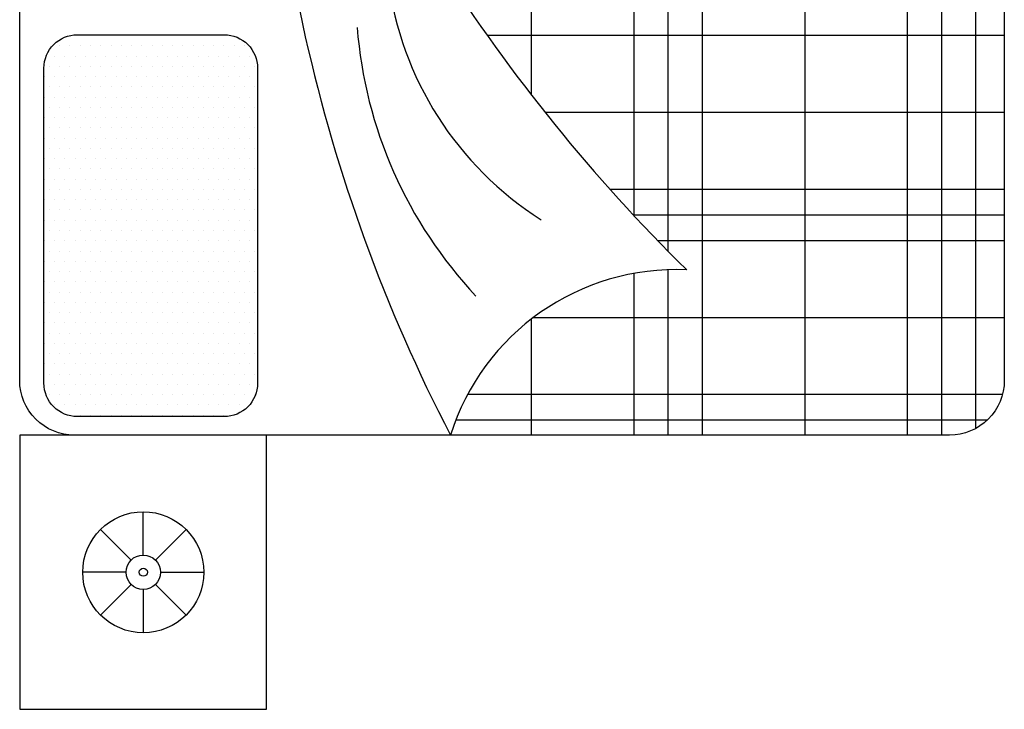
# Model space of a CAD drawing. Units: inches. Extents: x 528 to 2520, y -151 to 1354.
# Tile 18 of 41: x 1137 to 1192, y 1151 to 1189. Entities that reach past the tile are written whole.
import ezdxf

# ---------------------------------------------------------------- set-up
doc = ezdxf.new("R2010")
doc.units = ezdxf.units.IN
doc.header["$MEASUREMENT"] = 0
doc.layers.add('A-FURN', color=8, linetype='Continuous', lineweight=18)
doc.layers.add('BLOCK', color=6, linetype='Continuous')

# ---------------------------------------------------------------- blocks, each defined once
blk = doc.blocks.new('*X15')
at = {"color": 0}
for p, q in [((276.598, 451.25), (280.51, 451.25)), ((275.455, 450.625), (280.51, 450.625)), ((274.411, 450), (280.51, 450)), ((265.51, 448.125), (267.634, 448.125)), ((271.723, 448.125), (280.51, 448.125)), ((265.51, 446.25), (268.465, 446.25)), ((269.519, 446.25), (280.51, 446.25)), ((265.51, 445.625), (268.531, 445.625)), ((268.866, 445.625), (280.51, 445.625)), ((265.51, 445), (280.51, 445)), ((265.51, 443.125), (280.51, 443.125)), ((265.51, 441.25), (280.51, 441.25)), ((265.51, 440.625), (280.51, 440.625)), ((265.634, 440), (280.386, 440))]:
    blk.add_line(p, q, dxfattribs=at)
blk = doc.blocks.new('*X16')
at = {"color": 0}
for p, q in [((280.312, 439.886), (280.312, 452.896)), ((278.906, 439.482), (278.906, 452.338)), ((277.5, 439.482), (277.5, 451.702)), ((277.031, 439.482), (277.031, 451.471)), ((276.562, 439.482), (276.562, 451.231)), ((275.156, 439.482), (275.156, 450.451)), ((265.781, 439.797), (265.781, 449.511)), ((273.75, 439.482), (273.75, 449.576)), ((266.25, 439.517), (266.25, 449.296)), ((273.281, 439.482), (273.281, 449.261)), ((272.812, 439.482), (272.812, 448.934)), ((267.656, 439.482), (267.656, 448.095)), ((271.406, 439.482), (271.406, 447.876)), ((270, 439.482), (270, 446.689)), ((269.531, 439.482), (269.531, 446.262)), ((269.062, 439.482), (269.062, 445.817))]:
    blk.add_line(p, q, dxfattribs=at)
blk = doc.blocks.new('*X17')
at = {"color": 0}
for p, q in [((266.4375, 457.03125), (266.4375, 457.03125)), ((266.8125, 457.03125), (266.8125, 457.03125)), ((267.1875, 457.03125), (267.1875, 457.03125)), ((267.5625, 457.03125), (267.5625, 457.03125)), ((267.9375, 457.03125), (267.9375, 457.03125)), ((268.3125, 457.03125), (268.3125, 457.03125)), ((268.6875, 457.03125), (268.6875, 457.03125)), ((269.0625, 457.03125), (269.0625, 457.03125)), ((269.4375, 457.03125), (269.4375, 457.03125)), ((269.8125, 457.03125), (269.8125, 457.03125)), ((270.1875, 457.03125), (270.1875, 457.03125)), ((270.5625, 457.03125), (270.5625, 457.03125)), ((270.9375, 457.03125), (270.9375, 457.03125)), ((271.3125, 457.03125), (271.3125, 457.03125)), ((271.6875, 457.03125), (271.6875, 457.03125)), ((272.0625, 457.03125), (272.0625, 457.03125)), ((266.0625, 456.84375), (266.0625, 456.84375)), ((266.25, 456.9375), (266.25, 456.9375)), ((266.4375, 456.84375), (266.4375, 456.84375)), ((266.625, 456.9375), (266.625, 456.9375)), ((266.8125, 456.84375), (266.8125, 456.84375)), ((267, 456.9375), (267, 456.9375)), ((267.1875, 456.84375), (267.1875, 456.84375)), ((267.375, 456.9375), (267.375, 456.9375)), ((267.5625, 456.84375), (267.5625, 456.84375)), ((267.75, 456.9375), (267.75, 456.9375)), ((267.9375, 456.84375), (267.9375, 456.84375)), ((268.125, 456.9375), (268.125, 456.9375)), ((268.3125, 456.84375), (268.3125, 456.84375)), ((268.5, 456.9375), (268.5, 456.9375)), ((268.6875, 456.84375), (268.6875, 456.84375)), ((268.875, 456.9375), (268.875, 456.9375)), ((269.0625, 456.84375), (269.0625, 456.84375)), ((269.25, 456.9375), (269.25, 456.9375)), ((269.4375, 456.84375), (269.4375, 456.84375)), ((269.625, 456.9375), (269.625, 456.9375)), ((269.8125, 456.84375), (269.8125, 456.84375)), ((270, 456.9375), (270, 456.9375)), ((270.1875, 456.84375), (270.1875, 456.84375)), ((270.375, 456.9375), (270.375, 456.9375)), ((270.5625, 456.84375), (270.5625, 456.84375)), ((270.75, 456.9375), (270.75, 456.9375)), ((270.9375, 456.84375), (270.9375, 456.84375)), ((271.125, 456.9375), (271.125, 456.9375)), ((271.3125, 456.84375), (271.3125, 456.84375)), ((271.5, 456.9375), (271.5, 456.9375)), ((271.6875, 456.84375), (271.6875, 456.84375)), ((271.875, 456.9375), (271.875, 456.9375)), ((272.0625, 456.84375), (272.0625, 456.84375)), ((272.25, 456.9375), (272.25, 456.9375)), ((272.4375, 456.84375), (272.4375, 456.84375)), ((266.25, 456.75), (266.25, 456.75)), ((266.625, 456.75), (266.625, 456.75)), ((267, 456.75), (267, 456.75)), ((267.375, 456.75), (267.375, 456.75)), ((267.75, 456.75), (267.75, 456.75)), ((268.125, 456.75), (268.125, 456.75)), ((268.5, 456.75), (268.5, 456.75)), ((268.875, 456.75), (268.875, 456.75)), ((269.25, 456.75), (269.25, 456.75)), ((269.625, 456.75), (269.625, 456.75)), ((270, 456.75), (270, 456.75)), ((270.375, 456.75), (270.375, 456.75)), ((270.75, 456.75), (270.75, 456.75)), ((271.125, 456.75), (271.125, 456.75)), ((271.5, 456.75), (271.5, 456.75)), ((271.875, 456.75), (271.875, 456.75)), ((272.25, 456.75), (272.25, 456.75)), ((272.625, 456.75), (272.625, 456.75)), ((265.875, 456.5625), (265.875, 456.5625)), ((266.0625, 456.65625), (266.0625, 456.65625)), ((266.25, 456.5625), (266.25, 456.5625)), ((266.4375, 456.65625), (266.4375, 456.65625)), ((266.625, 456.5625), (266.625, 456.5625)), ((266.8125, 456.65625), (266.8125, 456.65625)), ((267, 456.5625), (267, 456.5625)), ((267.1875, 456.65625), (267.1875, 456.65625)), ((267.375, 456.5625), (267.375, 456.5625)), ((267.5625, 456.65625), (267.5625, 456.65625)), ((267.75, 456.5625), (267.75, 456.5625)), ((267.9375, 456.65625), (267.9375, 456.65625)), ((268.125, 456.5625), (268.125, 456.5625)), ((268.3125, 456.65625), (268.3125, 456.65625)), ((268.5, 456.5625), (268.5, 456.5625)), ((268.6875, 456.65625), (268.6875, 456.65625)), ((268.875, 456.5625), (268.875, 456.5625)), ((269.0625, 456.65625), (269.0625, 456.65625)), ((269.25, 456.5625), (269.25, 456.5625)), ((269.4375, 456.65625), (269.4375, 456.65625)), ((269.625, 456.5625), (269.625, 456.5625)), ((269.8125, 456.65625), (269.8125, 456.65625)), ((270, 456.5625), (270, 456.5625)), ((270.1875, 456.65625), (270.1875, 456.65625)), ((270.375, 456.5625), (270.375, 456.5625)), ((270.5625, 456.65625), (270.5625, 456.65625)), ((270.75, 456.5625), (270.75, 456.5625)), ((270.9375, 456.65625), (270.9375, 456.65625)), ((271.125, 456.5625), (271.125, 456.5625)), ((271.3125, 456.65625), (271.3125, 456.65625)), ((271.5, 456.5625), (271.5, 456.5625)), ((271.6875, 456.65625), (271.6875, 456.65625)), ((271.875, 456.5625), (271.875, 456.5625)), ((272.0625, 456.65625), (272.0625, 456.65625)), ((272.25, 456.5625), (272.25, 456.5625)), ((272.4375, 456.65625), (272.4375, 456.65625)), ((272.625, 456.5625), (272.625, 456.5625)), ((265.875, 456.375), (265.875, 456.375)), ((266.0625, 456.46875), (266.0625, 456.46875)), ((266.25, 456.375), (266.25, 456.375)), ((266.4375, 456.46875), (266.4375, 456.46875)), ((266.625, 456.375), (266.625, 456.375)), ((266.8125, 456.46875), (266.8125, 456.46875)), ((267, 456.375), (267, 456.375)), ((267.1875, 456.46875), (267.1875, 456.46875)), ((267.375, 456.375), (267.375, 456.375)), ((267.5625, 456.46875), (267.5625, 456.46875)), ((267.75, 456.375), (267.75, 456.375)), ((267.9375, 456.46875), (267.9375, 456.46875)), ((268.125, 456.375), (268.125, 456.375)), ((268.3125, 456.46875), (268.3125, 456.46875)), ((268.5, 456.375), (268.5, 456.375)), ((268.6875, 456.46875), (268.6875, 456.46875)), ((268.875, 456.375), (268.875, 456.375)), ((269.0625, 456.46875), (269.0625, 456.46875)), ((269.25, 456.375), (269.25, 456.375)), ((269.4375, 456.46875), (269.4375, 456.46875)), ((269.625, 456.375), (269.625, 456.375)), ((269.8125, 456.46875), (269.8125, 456.46875)), ((270, 456.375), (270, 456.375)), ((270.1875, 456.46875), (270.1875, 456.46875)), ((270.375, 456.375), (270.375, 456.375)), ((270.5625, 456.46875), (270.5625, 456.46875)), ((270.75, 456.375), (270.75, 456.375)), ((270.9375, 456.46875), (270.9375, 456.46875)), ((271.125, 456.375), (271.125, 456.375)), ((271.3125, 456.46875), (271.3125, 456.46875)), ((271.5, 456.375), (271.5, 456.375)), ((271.6875, 456.46875), (271.6875, 456.46875)), ((271.875, 456.375), (271.875, 456.375)), ((272.0625, 456.46875), (272.0625, 456.46875)), ((272.25, 456.375), (272.25, 456.375)), ((272.4375, 456.46875), (272.4375, 456.46875)), ((272.625, 456.375), (272.625, 456.375)), ((272.8125, 456.46875), (272.8125, 456.46875)), ((265.875, 456.1875), (265.875, 456.1875)), ((266.0625, 456.28125), (266.0625, 456.28125)), ((266.25, 456.1875), (266.25, 456.1875)), ((266.4375, 456.28125), (266.4375, 456.28125)), ((266.625, 456.1875), (266.625, 456.1875)), ((266.8125, 456.28125), (266.8125, 456.28125)), ((267, 456.1875), (267, 456.1875)), ((267.1875, 456.28125), (267.1875, 456.28125)), ((267.375, 456.1875), (267.375, 456.1875)), ((267.5625, 456.28125), (267.5625, 456.28125)), ((267.75, 456.1875), (267.75, 456.1875)), ((267.9375, 456.28125), (267.9375, 456.28125)), ((268.125, 456.1875), (268.125, 456.1875)), ((268.3125, 456.28125), (268.3125, 456.28125)), ((268.5, 456.1875), (268.5, 456.1875)), ((268.6875, 456.28125), (268.6875, 456.28125)), ((268.875, 456.1875), (268.875, 456.1875)), ((269.0625, 456.28125), (269.0625, 456.28125)), ((269.25, 456.1875), (269.25, 456.1875)), ((269.4375, 456.28125), (269.4375, 456.28125)), ((269.625, 456.1875), (269.625, 456.1875)), ((269.8125, 456.28125), (269.8125, 456.28125)), ((270, 456.1875), (270, 456.1875)), ((270.1875, 456.28125), (270.1875, 456.28125)), ((270.375, 456.1875), (270.375, 456.1875)), ((270.5625, 456.28125), (270.5625, 456.28125)), ((270.75, 456.1875), (270.75, 456.1875)), ((270.9375, 456.28125), (270.9375, 456.28125)), ((271.125, 456.1875), (271.125, 456.1875)), ((271.3125, 456.28125), (271.3125, 456.28125)), ((271.5, 456.1875), (271.5, 456.1875)), ((271.6875, 456.28125), (271.6875, 456.28125)), ((271.875, 456.1875), (271.875, 456.1875)), ((272.0625, 456.28125), (272.0625, 456.28125)), ((272.25, 456.1875), (272.25, 456.1875)), ((272.4375, 456.28125), (272.4375, 456.28125)), ((272.625, 456.1875), (272.625, 456.1875)), ((272.8125, 456.28125), (272.8125, 456.28125)), ((265.875, 456), (265.875, 456)), ((266.0625, 456.09375), (266.0625, 456.09375)), ((266.25, 456), (266.25, 456)), ((266.4375, 456.09375), (266.4375, 456.09375)), ((266.625, 456), (266.625, 456)), ((266.8125, 456.09375), (266.8125, 456.09375)), ((267, 456), (267, 456)), ((267.1875, 456.09375), (267.1875, 456.09375)), ((267.375, 456), (267.375, 456)), ((267.5625, 456.09375), (267.5625, 456.09375)), ((267.75, 456), (267.75, 456)), ((267.9375, 456.09375), (267.9375, 456.09375)), ((268.125, 456), (268.125, 456)), ((268.3125, 456.09375), (268.3125, 456.09375)), ((268.5, 456), (268.5, 456)), ((268.6875, 456.09375), (268.6875, 456.09375)), ((268.875, 456), (268.875, 456)), ((269.0625, 456.09375), (269.0625, 456.09375)), ((269.25, 456), (269.25, 456)), ((269.4375, 456.09375), (269.4375, 456.09375)), ((269.625, 456), (269.625, 456)), ((269.8125, 456.09375), (269.8125, 456.09375)), ((270, 456), (270, 456)), ((270.1875, 456.09375), (270.1875, 456.09375)), ((270.375, 456), (270.375, 456)), ((270.5625, 456.09375), (270.5625, 456.09375)), ((270.75, 456), (270.75, 456)), ((270.9375, 456.09375), (270.9375, 456.09375)), ((271.125, 456), (271.125, 456)), ((271.3125, 456.09375), (271.3125, 456.09375)), ((271.5, 456), (271.5, 456)), ((271.6875, 456.09375), (271.6875, 456.09375)), ((271.875, 456), (271.875, 456)), ((272.0625, 456.09375), (272.0625, 456.09375)), ((272.25, 456), (272.25, 456)), ((272.4375, 456.09375), (272.4375, 456.09375)), ((272.625, 456), (272.625, 456)), ((272.8125, 456.09375), (272.8125, 456.09375)), ((265.875, 455.8125), (265.875, 455.8125)), ((266.0625, 455.90625), (266.0625, 455.90625)), ((266.25, 455.8125), (266.25, 455.8125)), ((266.4375, 455.90625), (266.4375, 455.90625)), ((266.625, 455.8125), (266.625, 455.8125)), ((266.8125, 455.90625), (266.8125, 455.90625)), ((267, 455.8125), (267, 455.8125)), ((267.1875, 455.90625), (267.1875, 455.90625)), ((267.375, 455.8125), (267.375, 455.8125)), ((267.5625, 455.90625), (267.5625, 455.90625)), ((267.75, 455.8125), (267.75, 455.8125)), ((267.9375, 455.90625), (267.9375, 455.90625)), ((268.125, 455.8125), (268.125, 455.8125)), ((268.3125, 455.90625), (268.3125, 455.90625)), ((268.5, 455.8125), (268.5, 455.8125)), ((268.6875, 455.90625), (268.6875, 455.90625)), ((268.875, 455.8125), (268.875, 455.8125)), ((269.0625, 455.90625), (269.0625, 455.90625)), ((269.25, 455.8125), (269.25, 455.8125)), ((269.4375, 455.90625), (269.4375, 455.90625)), ((269.625, 455.8125), (269.625, 455.8125)), ((269.8125, 455.90625), (269.8125, 455.90625)), ((270, 455.8125), (270, 455.8125)), ((270.1875, 455.90625), (270.1875, 455.90625)), ((270.375, 455.8125), (270.375, 455.8125)), ((270.5625, 455.90625), (270.5625, 455.90625)), ((270.75, 455.8125), (270.75, 455.8125)), ((270.9375, 455.90625), (270.9375, 455.90625)), ((271.125, 455.8125), (271.125, 455.8125)), ((271.3125, 455.90625), (271.3125, 455.90625)), ((271.5, 455.8125), (271.5, 455.8125)), ((271.6875, 455.90625), (271.6875, 455.90625)), ((271.875, 455.8125), (271.875, 455.8125)), ((272.0625, 455.90625), (272.0625, 455.90625)), ((272.25, 455.8125), (272.25, 455.8125)), ((272.4375, 455.90625), (272.4375, 455.90625)), ((272.625, 455.8125), (272.625, 455.8125)), ((272.8125, 455.90625), (272.8125, 455.90625)), ((265.875, 455.625), (265.875, 455.625)), ((266.0625, 455.71875), (266.0625, 455.71875)), ((266.25, 455.625), (266.25, 455.625)), ((266.4375, 455.71875), (266.4375, 455.71875)), ((266.625, 455.625), (266.625, 455.625)), ((266.8125, 455.71875), (266.8125, 455.71875)), ((267, 455.625), (267, 455.625)), ((267.1875, 455.71875), (267.1875, 455.71875)), ((267.375, 455.625), (267.375, 455.625)), ((267.5625, 455.71875), (267.5625, 455.71875)), ((267.75, 455.625), (267.75, 455.625)), ((267.9375, 455.71875), (267.9375, 455.71875)), ((268.125, 455.625), (268.125, 455.625)), ((268.3125, 455.71875), (268.3125, 455.71875)), ((268.5, 455.625), (268.5, 455.625)), ((268.6875, 455.71875), (268.6875, 455.71875)), ((268.875, 455.625), (268.875, 455.625)), ((269.0625, 455.71875), (269.0625, 455.71875)), ((269.25, 455.625), (269.25, 455.625)), ((269.4375, 455.71875), (269.4375, 455.71875)), ((269.625, 455.625), (269.625, 455.625)), ((269.8125, 455.71875), (269.8125, 455.71875)), ((270, 455.625), (270, 455.625)), ((270.1875, 455.71875), (270.1875, 455.71875)), ((270.375, 455.625), (270.375, 455.625)), ((270.5625, 455.71875), (270.5625, 455.71875)), ((270.75, 455.625), (270.75, 455.625)), ((270.9375, 455.71875), (270.9375, 455.71875)), ((271.125, 455.625), (271.125, 455.625)), ((271.3125, 455.71875), (271.3125, 455.71875)), ((271.5, 455.625), (271.5, 455.625)), ((271.6875, 455.71875), (271.6875, 455.71875)), ((271.875, 455.625), (271.875, 455.625)), ((272.0625, 455.71875), (272.0625, 455.71875)), ((272.25, 455.625), (272.25, 455.625)), ((272.4375, 455.71875), (272.4375, 455.71875)), ((272.625, 455.625), (272.625, 455.625)), ((272.8125, 455.71875), (272.8125, 455.71875)), ((265.875, 455.4375), (265.875, 455.4375)), ((266.0625, 455.53125), (266.0625, 455.53125)), ((266.25, 455.4375), (266.25, 455.4375)), ((266.4375, 455.53125), (266.4375, 455.53125)), ((266.625, 455.4375), (266.625, 455.4375)), ((266.8125, 455.53125), (266.8125, 455.53125)), ((267, 455.4375), (267, 455.4375)), ((267.1875, 455.53125), (267.1875, 455.53125)), ((267.375, 455.4375), (267.375, 455.4375)), ((267.5625, 455.53125), (267.5625, 455.53125)), ((267.75, 455.4375), (267.75, 455.4375)), ((267.9375, 455.53125), (267.9375, 455.53125)), ((268.125, 455.4375), (268.125, 455.4375)), ((268.3125, 455.53125), (268.3125, 455.53125)), ((268.5, 455.4375), (268.5, 455.4375)), ((268.6875, 455.53125), (268.6875, 455.53125)), ((268.875, 455.4375), (268.875, 455.4375)), ((269.0625, 455.53125), (269.0625, 455.53125)), ((269.25, 455.4375), (269.25, 455.4375)), ((269.4375, 455.53125), (269.4375, 455.53125)), ((269.625, 455.4375), (269.625, 455.4375)), ((269.8125, 455.53125), (269.8125, 455.53125)), ((270, 455.4375), (270, 455.4375)), ((270.1875, 455.53125), (270.1875, 455.53125)), ((270.375, 455.4375), (270.375, 455.4375)), ((270.5625, 455.53125), (270.5625, 455.53125)), ((270.75, 455.4375), (270.75, 455.4375)), ((270.9375, 455.53125), (270.9375, 455.53125)), ((271.125, 455.4375), (271.125, 455.4375)), ((271.3125, 455.53125), (271.3125, 455.53125)), ((271.5, 455.4375), (271.5, 455.4375)), ((271.6875, 455.53125), (271.6875, 455.53125)), ((271.875, 455.4375), (271.875, 455.4375)), ((272.0625, 455.53125), (272.0625, 455.53125)), ((272.25, 455.4375), (272.25, 455.4375)), ((272.4375, 455.53125), (272.4375, 455.53125)), ((272.625, 455.4375), (272.625, 455.4375)), ((272.8125, 455.53125), (272.8125, 455.53125)), ((265.875, 455.25), (265.875, 455.25)), ((266.0625, 455.34375), (266.0625, 455.34375)), ((266.25, 455.25), (266.25, 455.25)), ((266.4375, 455.34375), (266.4375, 455.34375)), ((266.625, 455.25), (266.625, 455.25)), ((266.8125, 455.34375), (266.8125, 455.34375)), ((267, 455.25), (267, 455.25)), ((267.1875, 455.34375), (267.1875, 455.34375)), ((267.375, 455.25), (267.375, 455.25)), ((267.5625, 455.34375), (267.5625, 455.34375)), ((267.75, 455.25), (267.75, 455.25)), ((267.9375, 455.34375), (267.9375, 455.34375)), ((268.125, 455.25), (268.125, 455.25)), ((268.3125, 455.34375), (268.3125, 455.34375)), ((268.5, 455.25), (268.5, 455.25)), ((268.6875, 455.34375), (268.6875, 455.34375)), ((268.875, 455.25), (268.875, 455.25)), ((269.0625, 455.34375), (269.0625, 455.34375)), ((269.25, 455.25), (269.25, 455.25)), ((269.4375, 455.34375), (269.4375, 455.34375)), ((269.625, 455.25), (269.625, 455.25)), ((269.8125, 455.34375), (269.8125, 455.34375)), ((270, 455.25), (270, 455.25)), ((270.1875, 455.34375), (270.1875, 455.34375)), ((270.375, 455.25), (270.375, 455.25)), ((270.5625, 455.34375), (270.5625, 455.34375)), ((270.75, 455.25), (270.75, 455.25)), ((270.9375, 455.34375), (270.9375, 455.34375)), ((271.125, 455.25), (271.125, 455.25)), ((271.3125, 455.34375), (271.3125, 455.34375)), ((271.5, 455.25), (271.5, 455.25)), ((271.6875, 455.34375), (271.6875, 455.34375)), ((271.875, 455.25), (271.875, 455.25)), ((272.0625, 455.34375), (272.0625, 455.34375)), ((272.25, 455.25), (272.25, 455.25)), ((272.4375, 455.34375), (272.4375, 455.34375)), ((272.625, 455.25), (272.625, 455.25)), ((272.8125, 455.34375), (272.8125, 455.34375)), ((265.875, 455.0625), (265.875, 455.0625)), ((266.0625, 455.15625), (266.0625, 455.15625)), ((266.25, 455.0625), (266.25, 455.0625)), ((266.4375, 455.15625), (266.4375, 455.15625)), ((266.625, 455.0625), (266.625, 455.0625)), ((266.8125, 455.15625), (266.8125, 455.15625)), ((267, 455.0625), (267, 455.0625)), ((267.1875, 455.15625), (267.1875, 455.15625)), ((267.375, 455.0625), (267.375, 455.0625)), ((267.5625, 455.15625), (267.5625, 455.15625)), ((267.75, 455.0625), (267.75, 455.0625)), ((267.9375, 455.15625), (267.9375, 455.15625)), ((268.125, 455.0625), (268.125, 455.0625)), ((268.3125, 455.15625), (268.3125, 455.15625)), ((268.5, 455.0625), (268.5, 455.0625)), ((268.6875, 455.15625), (268.6875, 455.15625)), ((268.875, 455.0625), (268.875, 455.0625)), ((269.0625, 455.15625), (269.0625, 455.15625)), ((269.25, 455.0625), (269.25, 455.0625)), ((269.4375, 455.15625), (269.4375, 455.15625)), ((269.625, 455.0625), (269.625, 455.0625)), ((269.8125, 455.15625), (269.8125, 455.15625)), ((270, 455.0625), (270, 455.0625)), ((270.1875, 455.15625), (270.1875, 455.15625)), ((270.375, 455.0625), (270.375, 455.0625)), ((270.5625, 455.15625), (270.5625, 455.15625)), ((270.75, 455.0625), (270.75, 455.0625)), ((270.9375, 455.15625), (270.9375, 455.15625)), ((271.125, 455.0625), (271.125, 455.0625)), ((271.3125, 455.15625), (271.3125, 455.15625)), ((271.5, 455.0625), (271.5, 455.0625)), ((271.6875, 455.15625), (271.6875, 455.15625)), ((271.875, 455.0625), (271.875, 455.0625)), ((272.0625, 455.15625), (272.0625, 455.15625)), ((272.25, 455.0625), (272.25, 455.0625)), ((272.4375, 455.15625), (272.4375, 455.15625)), ((272.625, 455.0625), (272.625, 455.0625)), ((272.8125, 455.15625), (272.8125, 455.15625)), ((265.875, 454.875), (265.875, 454.875)), ((266.0625, 454.96875), (266.0625, 454.96875)), ((266.25, 454.875), (266.25, 454.875)), ((266.4375, 454.96875), (266.4375, 454.96875)), ((266.625, 454.875), (266.625, 454.875)), ((266.8125, 454.96875), (266.8125, 454.96875)), ((267, 454.875), (267, 454.875)), ((267.1875, 454.96875), (267.1875, 454.96875)), ((267.375, 454.875), (267.375, 454.875)), ((267.5625, 454.96875), (267.5625, 454.96875)), ((267.75, 454.875), (267.75, 454.875)), ((267.9375, 454.96875), (267.9375, 454.96875)), ((268.125, 454.875), (268.125, 454.875)), ((268.3125, 454.96875), (268.3125, 454.96875)), ((268.5, 454.875), (268.5, 454.875)), ((268.6875, 454.96875), (268.6875, 454.96875)), ((268.875, 454.875), (268.875, 454.875)), ((269.0625, 454.96875), (269.0625, 454.96875)), ((269.25, 454.875), (269.25, 454.875)), ((269.4375, 454.96875), (269.4375, 454.96875)), ((269.625, 454.875), (269.625, 454.875)), ((269.8125, 454.96875), (269.8125, 454.96875)), ((270, 454.875), (270, 454.875)), ((270.1875, 454.96875), (270.1875, 454.96875)), ((270.375, 454.875), (270.375, 454.875)), ((270.5625, 454.96875), (270.5625, 454.96875)), ((270.75, 454.875), (270.75, 454.875)), ((270.9375, 454.96875), (270.9375, 454.96875)), ((271.125, 454.875), (271.125, 454.875)), ((271.3125, 454.96875), (271.3125, 454.96875)), ((271.5, 454.875), (271.5, 454.875)), ((271.6875, 454.96875), (271.6875, 454.96875)), ((271.875, 454.875), (271.875, 454.875)), ((272.0625, 454.96875), (272.0625, 454.96875)), ((272.25, 454.875), (272.25, 454.875)), ((272.4375, 454.96875), (272.4375, 454.96875)), ((272.625, 454.875), (272.625, 454.875)), ((272.8125, 454.96875), (272.8125, 454.96875)), ((265.875, 454.6875), (265.875, 454.6875)), ((266.0625, 454.78125), (266.0625, 454.78125)), ((266.25, 454.6875), (266.25, 454.6875)), ((266.4375, 454.78125), (266.4375, 454.78125)), ((266.625, 454.6875), (266.625, 454.6875)), ((266.8125, 454.78125), (266.8125, 454.78125)), ((267, 454.6875), (267, 454.6875)), ((267.1875, 454.78125), (267.1875, 454.78125)), ((267.375, 454.6875), (267.375, 454.6875)), ((267.5625, 454.78125), (267.5625, 454.78125)), ((267.75, 454.6875), (267.75, 454.6875)), ((267.9375, 454.78125), (267.9375, 454.78125)), ((268.125, 454.6875), (268.125, 454.6875)), ((268.3125, 454.78125), (268.3125, 454.78125)), ((268.5, 454.6875), (268.5, 454.6875)), ((268.6875, 454.78125), (268.6875, 454.78125)), ((268.875, 454.6875), (268.875, 454.6875)), ((269.0625, 454.78125), (269.0625, 454.78125)), ((269.25, 454.6875), (269.25, 454.6875)), ((269.4375, 454.78125), (269.4375, 454.78125)), ((269.625, 454.6875), (269.625, 454.6875)), ((269.8125, 454.78125), (269.8125, 454.78125)), ((270, 454.6875), (270, 454.6875)), ((270.1875, 454.78125), (270.1875, 454.78125)), ((270.375, 454.6875), (270.375, 454.6875)), ((270.5625, 454.78125), (270.5625, 454.78125)), ((270.75, 454.6875), (270.75, 454.6875)), ((270.9375, 454.78125), (270.9375, 454.78125)), ((271.125, 454.6875), (271.125, 454.6875)), ((271.3125, 454.78125), (271.3125, 454.78125)), ((271.5, 454.6875), (271.5, 454.6875)), ((271.6875, 454.78125), (271.6875, 454.78125)), ((271.875, 454.6875), (271.875, 454.6875)), ((272.0625, 454.78125), (272.0625, 454.78125)), ((272.25, 454.6875), (272.25, 454.6875)), ((272.4375, 454.78125), (272.4375, 454.78125)), ((272.625, 454.6875), (272.625, 454.6875)), ((272.8125, 454.78125), (272.8125, 454.78125)), ((266.0625, 454.59375), (266.0625, 454.59375)), ((266.4375, 454.59375), (266.4375, 454.59375)), ((266.8125, 454.59375), (266.8125, 454.59375)), ((267.1875, 454.59375), (267.1875, 454.59375)), ((267.5625, 454.59375), (267.5625, 454.59375)), ((267.9375, 454.59375), (267.9375, 454.59375)), ((268.3125, 454.59375), (268.3125, 454.59375)), ((268.6875, 454.59375), (268.6875, 454.59375)), ((269.0625, 454.59375), (269.0625, 454.59375)), ((269.4375, 454.59375), (269.4375, 454.59375)), ((269.8125, 454.59375), (269.8125, 454.59375)), ((270.1875, 454.59375), (270.1875, 454.59375)), ((270.5625, 454.59375), (270.5625, 454.59375)), ((270.9375, 454.59375), (270.9375, 454.59375)), ((271.3125, 454.59375), (271.3125, 454.59375)), ((271.6875, 454.59375), (271.6875, 454.59375)), ((272.0625, 454.59375), (272.0625, 454.59375)), ((272.4375, 454.59375), (272.4375, 454.59375)), ((272.8125, 454.59375), (272.8125, 454.59375)), ((265.875, 454.5), (265.875, 454.5)), ((266.0625, 454.40625), (266.0625, 454.40625)), ((266.25, 454.5), (266.25, 454.5)), ((266.4375, 454.40625), (266.4375, 454.40625)), ((266.625, 454.5), (266.625, 454.5)), ((266.8125, 454.40625), (266.8125, 454.40625)), ((267, 454.5), (267, 454.5)), ((267.1875, 454.40625), (267.1875, 454.40625)), ((267.375, 454.5), (267.375, 454.5)), ((267.5625, 454.40625), (267.5625, 454.40625)), ((267.75, 454.5), (267.75, 454.5)), ((267.9375, 454.40625), (267.9375, 454.40625)), ((268.125, 454.5), (268.125, 454.5)), ((268.3125, 454.40625), (268.3125, 454.40625)), ((268.5, 454.5), (268.5, 454.5)), ((268.6875, 454.40625), (268.6875, 454.40625)), ((268.875, 454.5), (268.875, 454.5)), ((269.0625, 454.40625), (269.0625, 454.40625)), ((269.25, 454.5), (269.25, 454.5)), ((269.4375, 454.40625), (269.4375, 454.40625)), ((269.625, 454.5), (269.625, 454.5)), ((269.8125, 454.40625), (269.8125, 454.40625)), ((270, 454.5), (270, 454.5)), ((270.1875, 454.40625), (270.1875, 454.40625)), ((270.375, 454.5), (270.375, 454.5)), ((270.5625, 454.40625), (270.5625, 454.40625)), ((270.75, 454.5), (270.75, 454.5)), ((270.9375, 454.40625), (270.9375, 454.40625)), ((271.125, 454.5), (271.125, 454.5)), ((271.3125, 454.40625), (271.3125, 454.40625)), ((271.5, 454.5), (271.5, 454.5)), ((271.6875, 454.40625), (271.6875, 454.40625)), ((271.875, 454.5), (271.875, 454.5)), ((272.0625, 454.40625), (272.0625, 454.40625)), ((272.25, 454.5), (272.25, 454.5)), ((272.4375, 454.40625), (272.4375, 454.40625)), ((272.625, 454.5), (272.625, 454.5)), ((272.8125, 454.40625), (272.8125, 454.40625)), ((265.875, 454.3125), (265.875, 454.3125)), ((266.0625, 454.21875), (266.0625, 454.21875)), ((266.25, 454.3125), (266.25, 454.3125)), ((266.4375, 454.21875), (266.4375, 454.21875)), ((266.625, 454.3125), (266.625, 454.3125)), ((266.8125, 454.21875), (266.8125, 454.21875)), ((267, 454.3125), (267, 454.3125)), ((267.1875, 454.21875), (267.1875, 454.21875)), ((267.375, 454.3125), (267.375, 454.3125)), ((267.5625, 454.21875), (267.5625, 454.21875)), ((267.75, 454.3125), (267.75, 454.3125)), ((267.9375, 454.21875), (267.9375, 454.21875)), ((268.125, 454.3125), (268.125, 454.3125)), ((268.3125, 454.21875), (268.3125, 454.21875)), ((268.5, 454.3125), (268.5, 454.3125)), ((268.6875, 454.21875), (268.6875, 454.21875)), ((268.875, 454.3125), (268.875, 454.3125)), ((269.0625, 454.21875), (269.0625, 454.21875)), ((269.25, 454.3125), (269.25, 454.3125)), ((269.4375, 454.21875), (269.4375, 454.21875)), ((269.625, 454.3125), (269.625, 454.3125)), ((269.8125, 454.21875), (269.8125, 454.21875)), ((270, 454.3125), (270, 454.3125)), ((270.1875, 454.21875), (270.1875, 454.21875)), ((270.375, 454.3125), (270.375, 454.3125)), ((270.5625, 454.21875), (270.5625, 454.21875)), ((270.75, 454.3125), (270.75, 454.3125)), ((270.9375, 454.21875), (270.9375, 454.21875)), ((271.125, 454.3125), (271.125, 454.3125)), ((271.3125, 454.21875), (271.3125, 454.21875)), ((271.5, 454.3125), (271.5, 454.3125)), ((271.6875, 454.21875), (271.6875, 454.21875)), ((271.875, 454.3125), (271.875, 454.3125)), ((272.0625, 454.21875), (272.0625, 454.21875)), ((272.25, 454.3125), (272.25, 454.3125)), ((272.4375, 454.21875), (272.4375, 454.21875)), ((272.625, 454.3125), (272.625, 454.3125)), ((272.8125, 454.21875), (272.8125, 454.21875)), ((265.875, 454.125), (265.875, 454.125)), ((266.0625, 454.03125), (266.0625, 454.03125)), ((266.25, 454.125), (266.25, 454.125)), ((266.4375, 454.03125), (266.4375, 454.03125)), ((266.625, 454.125), (266.625, 454.125)), ((266.8125, 454.03125), (266.8125, 454.03125)), ((267, 454.125), (267, 454.125)), ((267.1875, 454.03125), (267.1875, 454.03125)), ((267.375, 454.125), (267.375, 454.125)), ((267.5625, 454.03125), (267.5625, 454.03125)), ((267.75, 454.125), (267.75, 454.125)), ((267.9375, 454.03125), (267.9375, 454.03125)), ((268.125, 454.125), (268.125, 454.125)), ((268.3125, 454.03125), (268.3125, 454.03125)), ((268.5, 454.125), (268.5, 454.125)), ((268.6875, 454.03125), (268.6875, 454.03125)), ((268.875, 454.125), (268.875, 454.125)), ((269.0625, 454.03125), (269.0625, 454.03125)), ((269.25, 454.125), (269.25, 454.125)), ((269.4375, 454.03125), (269.4375, 454.03125)), ((269.625, 454.125), (269.625, 454.125)), ((269.8125, 454.03125), (269.8125, 454.03125)), ((270, 454.125), (270, 454.125)), ((270.1875, 454.03125), (270.1875, 454.03125)), ((270.375, 454.125), (270.375, 454.125)), ((270.5625, 454.03125), (270.5625, 454.03125)), ((270.75, 454.125), (270.75, 454.125)), ((270.9375, 454.03125), (270.9375, 454.03125)), ((271.125, 454.125), (271.125, 454.125)), ((271.3125, 454.03125), (271.3125, 454.03125)), ((271.5, 454.125), (271.5, 454.125)), ((271.6875, 454.03125), (271.6875, 454.03125)), ((271.875, 454.125), (271.875, 454.125)), ((272.0625, 454.03125), (272.0625, 454.03125)), ((272.25, 454.125), (272.25, 454.125)), ((272.4375, 454.03125), (272.4375, 454.03125)), ((272.625, 454.125), (272.625, 454.125)), ((272.8125, 454.03125), (272.8125, 454.03125)), ((265.875, 453.9375), (265.875, 453.9375)), ((266.0625, 453.84375), (266.0625, 453.84375)), ((266.25, 453.9375), (266.25, 453.9375)), ((266.4375, 453.84375), (266.4375, 453.84375)), ((266.625, 453.9375), (266.625, 453.9375)), ((266.8125, 453.84375), (266.8125, 453.84375)), ((267, 453.9375), (267, 453.9375)), ((267.1875, 453.84375), (267.1875, 453.84375)), ((267.375, 453.9375), (267.375, 453.9375)), ((267.5625, 453.84375), (267.5625, 453.84375)), ((267.75, 453.9375), (267.75, 453.9375)), ((267.9375, 453.84375), (267.9375, 453.84375)), ((268.125, 453.9375), (268.125, 453.9375)), ((268.3125, 453.84375), (268.3125, 453.84375)), ((268.5, 453.9375), (268.5, 453.9375)), ((268.6875, 453.84375), (268.6875, 453.84375)), ((268.875, 453.9375), (268.875, 453.9375)), ((269.0625, 453.84375), (269.0625, 453.84375)), ((269.25, 453.9375), (269.25, 453.9375)), ((269.4375, 453.84375), (269.4375, 453.84375)), ((269.625, 453.9375), (269.625, 453.9375)), ((269.8125, 453.84375), (269.8125, 453.84375)), ((270, 453.9375), (270, 453.9375)), ((270.1875, 453.84375), (270.1875, 453.84375)), ((270.375, 453.9375), (270.375, 453.9375)), ((270.5625, 453.84375), (270.5625, 453.84375)), ((270.75, 453.9375), (270.75, 453.9375)), ((270.9375, 453.84375), (270.9375, 453.84375)), ((271.125, 453.9375), (271.125, 453.9375)), ((271.3125, 453.84375), (271.3125, 453.84375)), ((271.5, 453.9375), (271.5, 453.9375)), ((271.6875, 453.84375), (271.6875, 453.84375)), ((271.875, 453.9375), (271.875, 453.9375)), ((272.0625, 453.84375), (272.0625, 453.84375)), ((272.25, 453.9375), (272.25, 453.9375)), ((272.4375, 453.84375), (272.4375, 453.84375)), ((272.625, 453.9375), (272.625, 453.9375)), ((272.8125, 453.84375), (272.8125, 453.84375)), ((265.875, 453.75), (265.875, 453.75)), ((266.0625, 453.65625), (266.0625, 453.65625)), ((266.25, 453.75), (266.25, 453.75)), ((266.4375, 453.65625), (266.4375, 453.65625)), ((266.625, 453.75), (266.625, 453.75)), ((266.8125, 453.65625), (266.8125, 453.65625)), ((267, 453.75), (267, 453.75)), ((267.1875, 453.65625), (267.1875, 453.65625)), ((267.375, 453.75), (267.375, 453.75)), ((267.5625, 453.65625), (267.5625, 453.65625)), ((267.75, 453.75), (267.75, 453.75)), ((267.9375, 453.65625), (267.9375, 453.65625)), ((268.125, 453.75), (268.125, 453.75)), ((268.3125, 453.65625), (268.3125, 453.65625)), ((268.5, 453.75), (268.5, 453.75)), ((268.6875, 453.65625), (268.6875, 453.65625)), ((268.875, 453.75), (268.875, 453.75)), ((269.0625, 453.65625), (269.0625, 453.65625)), ((269.25, 453.75), (269.25, 453.75)), ((269.4375, 453.65625), (269.4375, 453.65625)), ((269.625, 453.75), (269.625, 453.75)), ((269.8125, 453.65625), (269.8125, 453.65625)), ((270, 453.75), (270, 453.75)), ((270.1875, 453.65625), (270.1875, 453.65625)), ((270.375, 453.75), (270.375, 453.75)), ((270.5625, 453.65625), (270.5625, 453.65625)), ((270.75, 453.75), (270.75, 453.75)), ((270.9375, 453.65625), (270.9375, 453.65625)), ((271.125, 453.75), (271.125, 453.75)), ((271.3125, 453.65625), (271.3125, 453.65625)), ((271.5, 453.75), (271.5, 453.75)), ((271.6875, 453.65625), (271.6875, 453.65625)), ((271.875, 453.75), (271.875, 453.75)), ((272.0625, 453.65625), (272.0625, 453.65625)), ((272.25, 453.75), (272.25, 453.75)), ((272.4375, 453.65625), (272.4375, 453.65625)), ((272.625, 453.75), (272.625, 453.75)), ((272.8125, 453.65625), (272.8125, 453.65625)), ((266.0625, 453.46875), (266.0625, 453.46875)), ((266.25, 453.5625), (266.25, 453.5625)), ((266.4375, 453.46875), (266.4375, 453.46875)), ((266.625, 453.5625), (266.625, 453.5625)), ((266.8125, 453.46875), (266.8125, 453.46875)), ((267, 453.5625), (267, 453.5625)), ((267.1875, 453.46875), (267.1875, 453.46875)), ((267.375, 453.5625), (267.375, 453.5625)), ((267.5625, 453.46875), (267.5625, 453.46875)), ((267.75, 453.5625), (267.75, 453.5625)), ((267.9375, 453.46875), (267.9375, 453.46875)), ((268.125, 453.5625), (268.125, 453.5625)), ((268.3125, 453.46875), (268.3125, 453.46875)), ((268.5, 453.5625), (268.5, 453.5625)), ((268.6875, 453.46875), (268.6875, 453.46875)), ((268.875, 453.5625), (268.875, 453.5625)), ((269.0625, 453.46875), (269.0625, 453.46875)), ((269.25, 453.5625), (269.25, 453.5625)), ((269.4375, 453.46875), (269.4375, 453.46875)), ((269.625, 453.5625), (269.625, 453.5625)), ((269.8125, 453.46875), (269.8125, 453.46875)), ((270, 453.5625), (270, 453.5625)), ((270.1875, 453.46875), (270.1875, 453.46875)), ((270.375, 453.5625), (270.375, 453.5625)), ((270.5625, 453.46875), (270.5625, 453.46875)), ((270.75, 453.5625), (270.75, 453.5625)), ((270.9375, 453.46875), (270.9375, 453.46875)), ((271.125, 453.5625), (271.125, 453.5625)), ((271.3125, 453.46875), (271.3125, 453.46875)), ((271.5, 453.5625), (271.5, 453.5625)), ((271.6875, 453.46875), (271.6875, 453.46875)), ((271.875, 453.5625), (271.875, 453.5625)), ((272.0625, 453.46875), (272.0625, 453.46875)), ((272.25, 453.5625), (272.25, 453.5625)), ((272.4375, 453.46875), (272.4375, 453.46875)), ((272.625, 453.5625), (272.625, 453.5625)), ((266.0625, 453.28125), (266.0625, 453.28125)), ((266.25, 453.375), (266.25, 453.375)), ((266.4375, 453.28125), (266.4375, 453.28125)), ((266.625, 453.375), (266.625, 453.375)), ((266.8125, 453.28125), (266.8125, 453.28125)), ((267, 453.375), (267, 453.375)), ((267.1875, 453.28125), (267.1875, 453.28125)), ((267.375, 453.375), (267.375, 453.375)), ((267.5625, 453.28125), (267.5625, 453.28125)), ((267.75, 453.375), (267.75, 453.375)), ((267.9375, 453.28125), (267.9375, 453.28125)), ((268.125, 453.375), (268.125, 453.375)), ((268.3125, 453.28125), (268.3125, 453.28125)), ((268.5, 453.375), (268.5, 453.375)), ((268.6875, 453.28125), (268.6875, 453.28125)), ((268.875, 453.375), (268.875, 453.375)), ((269.0625, 453.28125), (269.0625, 453.28125)), ((269.25, 453.375), (269.25, 453.375)), ((269.4375, 453.28125), (269.4375, 453.28125)), ((269.625, 453.375), (269.625, 453.375)), ((269.8125, 453.28125), (269.8125, 453.28125)), ((270, 453.375), (270, 453.375)), ((270.1875, 453.28125), (270.1875, 453.28125)), ((270.375, 453.375), (270.375, 453.375)), ((270.5625, 453.28125), (270.5625, 453.28125)), ((270.75, 453.375), (270.75, 453.375)), ((270.9375, 453.28125), (270.9375, 453.28125)), ((271.125, 453.375), (271.125, 453.375)), ((271.3125, 453.28125), (271.3125, 453.28125)), ((271.5, 453.375), (271.5, 453.375)), ((271.6875, 453.28125), (271.6875, 453.28125)), ((271.875, 453.375), (271.875, 453.375)), ((272.0625, 453.28125), (272.0625, 453.28125)), ((272.25, 453.375), (272.25, 453.375)), ((272.4375, 453.28125), (272.4375, 453.28125)), ((272.625, 453.375), (272.625, 453.375)), ((266.25, 453.1875), (266.25, 453.1875)), ((266.625, 453.1875), (266.625, 453.1875)), ((267, 453.1875), (267, 453.1875)), ((267.375, 453.1875), (267.375, 453.1875)), ((267.75, 453.1875), (267.75, 453.1875)), ((268.125, 453.1875), (268.125, 453.1875)), ((268.5, 453.1875), (268.5, 453.1875)), ((268.875, 453.1875), (268.875, 453.1875)), ((269.25, 453.1875), (269.25, 453.1875)), ((269.625, 453.1875), (269.625, 453.1875)), ((270, 453.1875), (270, 453.1875)), ((270.375, 453.1875), (270.375, 453.1875)), ((270.75, 453.1875), (270.75, 453.1875)), ((271.125, 453.1875), (271.125, 453.1875)), ((271.5, 453.1875), (271.5, 453.1875)), ((271.875, 453.1875), (271.875, 453.1875)), ((272.25, 453.1875), (272.25, 453.1875))]:
    blk.add_line(p, q, dxfattribs=at)
blk = doc.blocks.new('A$C52E67D0D')
at = {"layer": 'BLOCK'}
for p, q in [((250.5, 1605.5), (250.5, 1684.7)), ((228.3, 1596.3), (172.3, 1652.3)), ((272.7, 1596.3), (328.7, 1652.3)), ((219.1, 1574.1), (139.9, 1574.1)), ((281.9, 1574.1), (361.1, 1574.1)), ((228.3, 1551.9), (172.3, 1495.9)), ((272.7, 1551.9), (328.7, 1495.9)), ((250.5, 1542.8), (250.5, 1463.5))]:
    blk.add_line(p, q, dxfattribs=at)
for points in [[(1901, 0), (601, 0, -0.414214), (501, 100), (501, 1700, -0.414214), (601, 1800), (1901, 1800, -0.414214), (2001, 1700), (2001, 100, -0.414214)], [(1171.8, 1365.1), (595.8, 1365.1, -0.414214), (535, 1425.9), (535, 1694.8, -0.414214), (595.8, 1755.7), (1171.8, 1755.7, -0.414214), (1232.6, 1694.8), (1232.6, 1425.9, -0.414214)]]:
    blk.add_lwpolyline(points, format="xyb", close=True, dxfattribs=at)
blk.add_lwpolyline([(501, 1348.6), (501, 1799.6), (0, 1799.6), (0, 1348.6)], close=True, dxfattribs=at)
for radius in [110.6, 31.4, 7.46]:
    blk.add_circle((250.5, 1574.1), radius, dxfattribs=at)
for centre, radius, start, end in [((1888.6, -1664.5), 3015.3, 87.8642, 117.4001), ((3101, -1685.8), 3227.7, 109.926, 135.3977), ((1308.8, 377.9), 807.6, 94.4436, 133.2788), ((1410.8, 520.2), 610.8, 97.2157, 147.6656), ((371.4, 600.4), 432, 357.3792, 72.5379)]:
    blk.add_arc(centre, radius, start, end, dxfattribs=at)
at = {"layer": 'BLOCK', "xscale": 100, "yscale": 100, "zscale": 100}
for name in ['*X17', '*X16', '*X15']:
    blk.add_blockref(name, (-26050, -43948.2), dxfattribs=at)

msp = doc.modelspace()

# ---------------------------------------------------------------- block references
at = {"layer": 'A-FURN', "xscale": 0.0306954436450662, "yscale": 0.0306954436450662, "zscale": 0.0306954436450662, "rotation": 90}
msp.add_blockref('A$C52E67D0D', (1192.308, 1150.631), dxfattribs=at)

doc.saveas('drawing.dxf')
